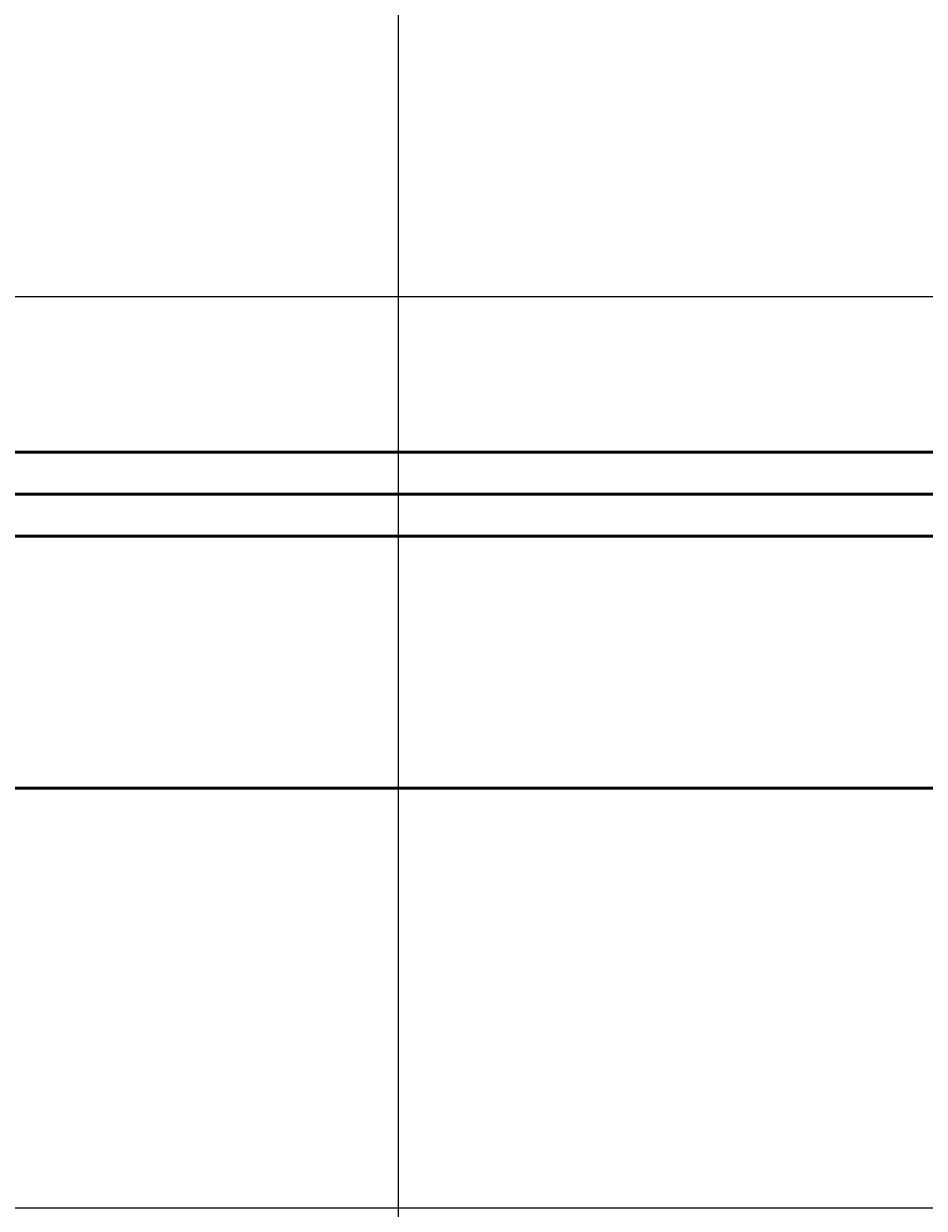
# Model space of a CAD drawing. Units: inches. Extents: x 2812 to 3051, y 1398 to 1659.
# Tile 24 of 65: x 2902 to 2923, y 1472 to 1500. Entities that reach past the tile are written whole.
import ezdxf

# ---------------------------------------------------------------- set-up
doc = ezdxf.new("R2010")
doc.units = ezdxf.units.IN
doc.layers.add('A-ANNO-DIMS', color=2, linetype='Continuous', lineweight=18)
doc.layers.add('S-CONC', color=7, linetype='Continuous', lineweight=50)
doc.styles.get("Standard").update_dxf_attribs({"font": 'arial.ttf'})
doc.dimstyles.get("Standard").update_dxf_attribs({"dimtxt": 0.18, "dimasz": 0.18, "dimexe": 0.18, "dimexo": 0.0625, "dimgap": 0.09, "dimtad": 0, "dimtih": 1, "dimtoh": 1, "dimdec": 4, "dimzin": 0, "dimdsep": 46, "dimtxsty": 'Standard', "dimcen": 0.09, "dimadec": 0, "dimazin": 0, "dimtfac": 1, "dimtdec": 4, "dimtofl": 0, "dimtmove": 0, "dimatfit": 3, "dimfxl": 1, "dimtolj": 1, "dimtzin": 0, "dimarcsym": 0})

# ---------------------------------------------------------------- blocks, each defined once
blk = doc.blocks.new('*D29')
at = {"layer": 'A-ANNO-DIMS', "color": 0, "lineweight": -2, "transparency": 16777216}
for p, q in [((2910.742, 1598.757), (2910.742, 1397.505)), ((2883.385, 1559.757), (2883.385, 1397.505)), ((2883.565, 1397.685), (2896.598, 1397.685)), ((2910.562, 1397.685), (2897.528, 1397.685))]:
    blk.add_line(p, q, dxfattribs=at)
at = {"layer": 'A-ANNO-DIMS', "color": 0, "transparency": 16777216}
for points in [[(2883.565, 1397.715), (2883.565, 1397.655), (2883.385, 1397.685)], [(2910.562, 1397.715), (2910.562, 1397.655), (2910.742, 1397.685)]]:
    blk.add_solid(points, dxfattribs=at)
at = {"layer": 'Defpoints', "color": 0, "transparency": 16777216}
for p in [(2910.742, 1598.82), (2883.385, 1559.82), (2910.742, 1397.685)]:
    blk.add_point(p, dxfattribs=at)
at = {"layer": 'A-ANNO-DIMS', "color": 0, "transparency": 16777216, "insert": (2897.063, 1397.685), "char_height": 0.18, "attachment_point": 5}
blk.add_mtext('\\A1;27.357', dxfattribs=at)
blk = doc.blocks.new('*D45')
at = {"layer": 'A-ANNO-DIMS', "color": 0, "lineweight": -2, "transparency": 16777216}
for p, q in [((2896.385, 1487.973), (2896.385, 1397.505)), ((2941.385, 1487.973), (2941.385, 1397.505)), ((2896.565, 1397.685), (2918.662, 1397.685)), ((2941.205, 1397.685), (2919.108, 1397.685))]:
    blk.add_line(p, q, dxfattribs=at)
at = {"layer": 'A-ANNO-DIMS', "color": 0, "transparency": 16777216}
for points in [[(2896.565, 1397.715), (2896.565, 1397.655), (2896.385, 1397.685)], [(2941.205, 1397.715), (2941.205, 1397.655), (2941.385, 1397.685)]]:
    blk.add_solid(points, dxfattribs=at)
at = {"layer": 'Defpoints', "color": 0, "transparency": 16777216}
for p in [(2896.385, 1488.035), (2941.385, 1488.035), (2941.385, 1397.685)]:
    blk.add_point(p, dxfattribs=at)
at = {"layer": 'A-ANNO-DIMS', "color": 0, "transparency": 16777216, "insert": (2918.885, 1397.685), "char_height": 0.18, "attachment_point": 5}
blk.add_mtext('\\A1;45', dxfattribs=at)
blk = doc.blocks.new('*D55')
at = {"layer": 'A-ANNO-DIMS', "color": 0, "lineweight": -2, "transparency": 16777216}
for p, q in [((2850.811, 1493.738), (3051.178, 1493.738)), ((3050.998, 1493.558), (3050.998, 1491.069)), ((3050.998, 1488.215), (3050.998, 1490.705)), ((2850.811, 1488.035), (3051.178, 1488.035))]:
    blk.add_line(p, q, dxfattribs=at)
at = {"layer": 'A-ANNO-DIMS', "color": 0, "transparency": 16777216}
for points in [[(3050.968, 1493.558), (3051.028, 1493.558), (3050.998, 1493.738)], [(3050.968, 1488.215), (3051.028, 1488.215), (3050.998, 1488.035)]]:
    blk.add_solid(points, dxfattribs=at)
at = {"layer": 'Defpoints', "color": 0, "transparency": 16777216}
for p in [(2850.748, 1493.738), (3050.998, 1493.738), (2850.748, 1488.035)]:
    blk.add_point(p, dxfattribs=at)
at = {"layer": 'A-ANNO-DIMS', "color": 0, "transparency": 16777216, "insert": (3050.998, 1490.887), "char_height": 0.18, "attachment_point": 5}
blk.add_mtext('\\A1;5.703', dxfattribs=at)
blk = doc.blocks.new('*D77')
at = {"layer": 'A-ANNO-DIMS', "color": 0, "lineweight": -2, "transparency": 16777216}
for p, q in [((2961.322, 1472.035), (2811.806, 1472.035)), ((2811.986, 1471.855), (2811.986, 1461.436)), ((2811.986, 1450.654), (2811.986, 1461.073)), ((2963.812, 1450.474), (2811.806, 1450.474))]:
    blk.add_line(p, q, dxfattribs=at)
at = {"layer": 'A-ANNO-DIMS', "color": 0, "transparency": 16777216}
for points in [[(2811.956, 1471.855), (2812.016, 1471.855), (2811.986, 1472.035)], [(2811.956, 1450.654), (2812.016, 1450.654), (2811.986, 1450.474)]]:
    blk.add_solid(points, dxfattribs=at)
at = {"layer": 'Defpoints', "color": 0, "transparency": 16777216}
for p in [(2811.986, 1472.035), (2961.385, 1472.035), (2963.874, 1450.474)]:
    blk.add_point(p, dxfattribs=at)
at = {"layer": 'A-ANNO-DIMS', "color": 0, "transparency": 16777216, "insert": (2811.986, 1461.255), "char_height": 0.18, "attachment_point": 5}
blk.add_mtext('\\A1;21.56', dxfattribs=at)

msp = doc.modelspace()

# ---------------------------------------------------------------- linework, layer by layer
at = {"layer": 'S-CONC'}
for p, q in [((3034.3849, 1490.0354), (2850.7485, 1490.0354)), ((2850.7485, 1489.0354), (3035.3849, 1489.0354)), ((2850.7485, 1488.0354), (3036.3849, 1488.0354)), ((2850.7485, 1482.0354), (3027.3849, 1482.0354))]:
    msp.add_line(p, q, dxfattribs=at)

# ---------------------------------------------------------------- dimensions: what is measured, and where the dimension line sits
at = {"layer": 'A-ANNO-DIMS'}
for base, p1, p2, override, picture, middle in [((2910.7415, 1397.6854), (2883.3849, 1559.82), (2910.7415, 1598.82), {"dimdec": 3, "dimlfac": 1, "dimrnd": 0, "dimzin": 0, "dimdsep": 46, "dimlunit": 2}, '*D29', (2897.0632, 1397.6854)), ((2941.3849, 1397.6854), (2896.3849, 1488.0354), (2941.3849, 1488.0354), {"dimdec": 0, "dimlfac": 1, "dimrnd": 0, "dimzin": 0, "dimdsep": 46, "dimlunit": 2}, '*D45', (2918.8849, 1397.6854))]:
    dim = msp.add_linear_dim(base=base, p1=p1, p2=p2, dimstyle='Standard', override=override, dxfattribs=at)
    dim.commit()
    dim.dimension.update_dxf_attribs({"geometry": picture, "text_midpoint": middle})
for base, p1, p2, override, picture, middle in [((3050.998, 1493.7383), (2850.7485, 1488.0354), (2850.7485, 1493.7383), {"dimdec": 3, "dimlfac": 1, "dimrnd": 0, "dimzin": 0, "dimdsep": 46, "dimlunit": 2}, '*D55', (3050.998, 1490.8868)), ((2811.9855, 1472.0354), (2963.8741, 1450.4738), (2961.3849, 1472.0354), {"dimdec": 2, "dimlfac": 1, "dimrnd": 0, "dimzin": 0, "dimdsep": 46, "dimlunit": 2}, '*D77', (2811.9855, 1461.2546))]:
    dim = msp.add_linear_dim(base=base, p1=p1, p2=p2, angle=90, dimstyle='Standard', override=override, dxfattribs=at)
    dim.commit()
    dim.dimension.update_dxf_attribs({"geometry": picture, "text_midpoint": middle})

doc.saveas('drawing.dxf')
